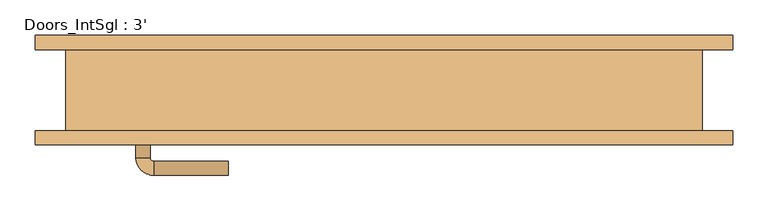
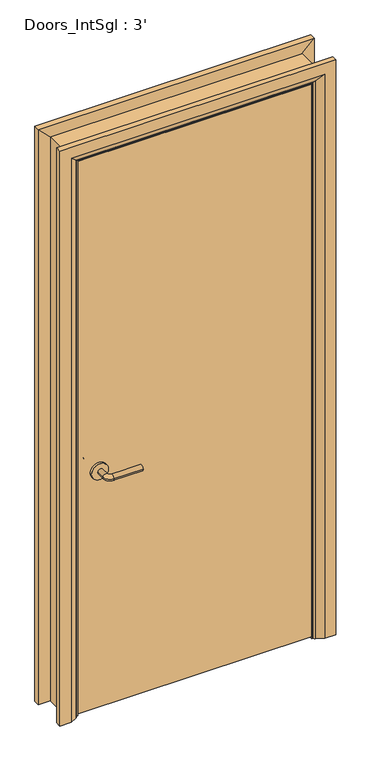
"""IFC4 building model written with IfcOpenShell, lengths in millimetres: door geometry, Doors_IntSgl : 3'."""

from ifc_helpers import new_model, si_unit, point, frame, frame_2d, origin, place, context, project, spatial, polyline, circle_curve, ellipse_curve, trimmed, segment, composite_curve, outline, extrude, faceted_brep, source, transform, mapped, element, save
from ifc_brep_helpers import plane_surface, cylinder_surface, revolved_surface, advanced_brep


def doors_intsgl_3_f3216364(model_context):
    return source(origin(), model_context, "Body", "SolidModel", [
        advanced_brep(
        [(-350.2, -11.15, 900.0), (-330.2, -11.15, 900.0), (-350.2, 18.85, 900.0), (-330.2, 18.85, 900.0), (-325.2, 23.85, 900.0), (-325.2, 43.85, 900.0), (-220.2, 43.85, 900.0), (-220.2, 23.85, 900.0)],
        [
            (0, 1, circle_curve(frame((-340.2, -11.15, 900.0), z_axis=(0.0, -1.0, 0.0), x_axis=(1.0, 0.0, 0.0)), 10.0)),
            (1, 0, circle_curve(frame((-340.2, -11.15, 900.0), z_axis=(0.0, -1.0, 0.0), x_axis=(1.0, 0.0, 0.0)), 10.0)),
            (0, 2),
            (2, 3, circle_curve(frame((-340.2, 18.85, 900.0), z_axis=(0.0, -1.0, 0.0), x_axis=(1.0, 0.0, 0.0)), 10.0)),
            (3, 1),
            (3, 2, circle_curve(frame((-340.2, 18.85, 900.0), z_axis=(0.0, -1.0, 0.0), x_axis=(1.0, 0.0, 0.0)), 10.0)),
            (4, 3, circle_curve(frame((-325.2, 18.85, 900.0), z_axis=(0.0, 0.0, 1.0), x_axis=(-1.0, 0.0, 0.0)), 5.0)),
            (2, 5, circle_curve(frame((-325.2, 18.85, 900.0), z_axis=(0.0, 0.0, -1.0), x_axis=(-1.0, 0.0, 0.0)), 25.0)),
            (5, 4, circle_curve(frame((-325.2, 33.85, 900.0), z_axis=(-1.0, 0.0, 0.0), x_axis=(0.0, -1.0, 0.0)), 10.0)),
            (4, 5, circle_curve(frame((-325.2, 33.85, 900.0), z_axis=(-1.0, 0.0, 0.0), x_axis=(0.0, -1.0, 0.0)), 10.0)),
            (6, 7, circle_curve(frame((-220.2, 33.85, 900.0), z_axis=(1.0, 0.0, 0.0), x_axis=(0.0, -1.0, 0.0)), 10.0)),
            (7, 6, circle_curve(frame((-220.2, 33.85, 900.0), z_axis=(1.0, 0.0, 0.0), x_axis=(0.0, -1.0, 0.0)), 10.0)),
            (5, 6),
            (7, 4),
        ],
        [
            plane_surface(frame((-340.2, -11.15, 900.0), z_axis=(0.0, -1.0, 0.0), x_axis=(0.0, 0.0, 1.0))),
            cylinder_surface(frame((-340.2, -11.15, 900.0), z_axis=(0.0, -1.0, 0.0), x_axis=(1.0, 0.0, 0.0)), 10.0),
            revolved_surface(trimmed(ellipse_curve(frame((-340.2, 18.85, 900.0), z_axis=(0.0, -1.0, 0.0), x_axis=(1.0, 0.0, 0.0)), 10.0, 10.0), [point((-350.2, 18.85, 900.0))], [point((-330.2, 18.85, 900.0))], True, "CARTESIAN"), (-325.2, 18.85, 900.0), (0.0, 0.0, -1.0)),
            revolved_surface(trimmed(ellipse_curve(frame((-340.2, 18.85, 900.0), z_axis=(0.0, -1.0, 0.0), x_axis=(1.0, 0.0, 0.0)), 10.0, 10.0), [point((-330.2, 18.85, 900.0))], [point((-350.2, 18.85, 900.0))], True, "CARTESIAN"), (-325.2, 18.85, 900.0), (0.0, 0.0, -1.0)),
            plane_surface(frame((-220.2, 33.85, 900.0), z_axis=(1.0, 0.0, 0.0), x_axis=(0.0, 0.0, 1.0))),
            cylinder_surface(frame((-325.2, 33.85, 900.0), z_axis=(-1.0, 0.0, 0.0), x_axis=(0.0, -1.0, 0.0)), 10.0),
        ],
        [
            (0, [[1, 2]]),
            (1, [[-1, 3, 4, 5]]),
            (1, [[-2, -5, 6, -3]]),
            (2, [[7, -4, 8, 9]]),
            (3, [[-8, -6, -7, 10]]),
            (4, [[11, 12]]),
            (5, [[-9, 13, -12, 14]]),
            (5, [[-10, -14, -11, -13]]),
        ],
    ),
        extrude(outline(composite_curve([segment(trimmed(circle_curve(frame_2d((900.0, -342.7)), 30.0), [point((900.0, -372.7))], [point((900.0, -312.7))], False, "CARTESIAN"), True, "CONTINUOUS"), segment(trimmed(circle_curve(frame_2d((900.0, -342.7)), 30.0), [point((900.0, -312.7))], [point((900.0, -372.7))], False, "CARTESIAN"), True, "CONTINUOUS")], self_intersect=False)), frame((0.0, -19.15, 0.0), z_axis=(0.0, 1.0, 0.0), x_axis=(0.0, 0.0, 1.0)), (0.0, 0.0, 1.0), 8.0),
        advanced_brep(
        [(-350.2, -65.15, 900.0), (-330.2, -65.15, 900.0), (-330.2, -95.15, 900.0), (-350.2, -95.15, 900.0), (-325.2, -100.15, 900.0), (-325.2, -120.15, 900.0), (-220.2, -120.15, 900.0), (-220.2, -100.15, 900.0)],
        [
            (0, 1, circle_curve(frame((-340.2, -65.15, 900.0), z_axis=(0.0, 1.0, 0.0), x_axis=(1.0, 0.0, 0.0)), 10.0)),
            (1, 0, circle_curve(frame((-340.2, -65.15, 900.0), z_axis=(0.0, 1.0, 0.0), x_axis=(1.0, 0.0, 0.0)), 10.0)),
            (1, 2),
            (2, 3, circle_curve(frame((-340.2, -95.15, 900.0), z_axis=(0.0, 1.0, 0.0), x_axis=(1.0, 0.0, 0.0)), 10.0)),
            (3, 0),
            (3, 2, circle_curve(frame((-340.2, -95.15, 900.0), z_axis=(0.0, 1.0, 0.0), x_axis=(1.0, 0.0, 0.0)), 10.0)),
            (4, 5, circle_curve(frame((-325.2, -110.15, 900.0), z_axis=(-1.0, 0.0, 0.0), x_axis=(0.0, 1.0, 0.0)), 10.0)),
            (5, 3, circle_curve(frame((-325.2, -95.15, 900.0), z_axis=(0.0, 0.0, -1.0), x_axis=(-1.0, 0.0, 0.0)), 25.0)),
            (2, 4, circle_curve(frame((-325.2, -95.15, 900.0), z_axis=(0.0, 0.0, 1.0), x_axis=(-1.0, 0.0, 0.0)), 5.0)),
            (5, 4, circle_curve(frame((-325.2, -110.15, 900.0), z_axis=(-1.0, 0.0, 0.0), x_axis=(0.0, 1.0, 0.0)), 10.0)),
            (6, 7, circle_curve(frame((-220.2, -110.15, 900.0), z_axis=(1.0, 0.0, 0.0), x_axis=(0.0, 1.0, 0.0)), 10.0)),
            (7, 6, circle_curve(frame((-220.2, -110.15, 900.0), z_axis=(1.0, 0.0, 0.0), x_axis=(0.0, 1.0, 0.0)), 10.0)),
            (4, 7),
            (6, 5),
        ],
        [
            plane_surface(frame((-340.2, -65.15, 900.0), z_axis=(0.0, 1.0, 0.0), x_axis=(0.0, 0.0, 1.0))),
            cylinder_surface(frame((-340.2, -65.15, 900.0), z_axis=(0.0, 1.0, 0.0), x_axis=(1.0, 0.0, 0.0)), 10.0),
            revolved_surface(trimmed(ellipse_curve(frame((-340.2, -95.15, 900.0), z_axis=(0.0, -1.0, 0.0), x_axis=(1.0, 0.0, 0.0)), 10.0, 10.0), [point((-350.2, -95.15, 900.0))], [point((-330.2, -95.15, 900.0))], True, "CARTESIAN"), (-325.2, -95.15, 900.0), (0.0, 0.0, -1.0)),
            revolved_surface(trimmed(ellipse_curve(frame((-340.2, -95.15, 900.0), z_axis=(0.0, -1.0, 0.0), x_axis=(1.0, 0.0, 0.0)), 10.0, 10.0), [point((-330.2, -95.15, 900.0))], [point((-350.2, -95.15, 900.0))], True, "CARTESIAN"), (-325.2, -95.15, 900.0), (0.0, 0.0, -1.0)),
            plane_surface(frame((-220.2, -110.15, 900.0), z_axis=(1.0, 0.0, 0.0), x_axis=(0.0, 0.0, 1.0))),
            cylinder_surface(frame((-325.2, -110.15, 900.0), z_axis=(-1.0, 0.0, 0.0), x_axis=(0.0, 1.0, 0.0)), 10.0),
        ],
        [
            (0, [[1, 2]]),
            (1, [[3, 4, 5, -2]]),
            (1, [[-5, 6, -3, -1]]),
            (2, [[7, 8, -4, 9]]),
            (3, [[10, -9, -6, -8]]),
            (4, [[11, 12]]),
            (5, [[13, -11, 14, -7]]),
            (5, [[-14, -12, -13, -10]]),
        ],
    ),
        extrude(outline(composite_curve([segment(trimmed(circle_curve(frame_2d((900.0, -342.7)), 30.0), [point((900.0, -372.7))], [point((900.0, -312.7))], False, "CARTESIAN"), True, "CONTINUOUS"), segment(trimmed(circle_curve(frame_2d((900.0, -342.7)), 30.0), [point((900.0, -312.7))], [point((900.0, -372.7))], False, "CARTESIAN"), True, "CONTINUOUS")], self_intersect=False)), frame((0.0, -65.15, 0.0), z_axis=(0.0, 1.0, 0.0), x_axis=(0.0, 0.0, 1.0)), (0.0, 0.0, 1.0), 8.0),
        extrude(outline(polyline([(415.2, -19.15), (415.2, -57.15), (-415.2, -57.15), (-415.2, -19.15), (415.2, -19.15)])), frame((0.0, 0.0, 8.0), z_axis=(0.0, 0.0, 1.0), x_axis=(1.0, 0.0, 0.0)), (0.0, 0.0, 1.0), 2083.6),
        advanced_brep(
        [(492.2, -77.15, 0.0), (452.2, -77.15, 0.0), (426.2, -63.15, 0.0), (422.2, -57.15, 0.0), (492.2, -57.15, 0.0), (492.2, -57.15, 2168.6), (492.2, -77.15, 2168.6), (422.2, -57.15, 2098.6), (-422.2, -57.15, 2098.6), (-422.2, -57.15, 0.0), (-492.2, -57.15, 0.0), (-492.2, -57.15, 2168.6), (426.2, -63.15, 2102.6), (452.2, -77.15, 2128.6), (-492.2, -77.15, 2168.6), (-492.2, -77.15, 0.0), (-452.2, -77.15, 0.0), (-452.2, -77.15, 2128.6), (-426.2, -63.15, 0.0), (-426.2, -63.15, 2102.6)],
        [
            (0, 1),
            (1, 2),
            (2, 3, circle_curve(frame((430.2, -56.15, 0.0), z_axis=(0.0, 0.0, -1.0), x_axis=(1.0, 0.0, 0.0)), 8.0622577)),
            (3, 4),
            (4, 0),
            (4, 5),
            (5, 6),
            (6, 0),
            (3, 7),
            (7, 8),
            (8, 9),
            (9, 10),
            (10, 11),
            (11, 5),
            (2, 12),
            (12, 7, ellipse_curve(frame((430.2, -56.15, 2106.6), z_axis=(0.7071067811865475, 0.0, -0.7071067811865475), x_axis=(-0.7071067811865474, 0.0, -0.7071067811865476)), 11.4017543, 8.0622577)),
            (1, 13),
            (13, 12),
            (6, 14),
            (14, 15),
            (15, 16),
            (16, 17),
            (17, 13),
            (10, 15),
            (14, 11),
            (9, 18, circle_curve(frame((-430.2, -56.15, 0.0), z_axis=(0.0, 0.0, -1.0), x_axis=(-1.0, 0.0, 0.0)), 8.0622577)),
            (18, 16),
            (19, 18),
            (8, 19, ellipse_curve(frame((-430.2, -56.15, 2106.6), z_axis=(-0.7071067811865475, 0.0, -0.7071067811865475), x_axis=(-0.7071067811865474, 0.0, 0.7071067811865476)), 11.4017543, 8.0622577)),
            (19, 17),
            (12, 19),
        ],
        [
            plane_surface(frame((422.2, -57.15, 0.0), z_axis=(0.0, 0.0, -1.0), x_axis=(0.0, 1.0, 0.0))),
            plane_surface(frame((492.2, -77.15, 0.0), z_axis=(1.0, 0.0, 0.0), x_axis=(0.0, 0.0, 1.0))),
            plane_surface(frame((492.2, -57.15, 0.0), z_axis=(0.0, 1.0, 0.0), x_axis=(0.0, 0.0, 1.0))),
            cylinder_surface(frame((430.2, -56.15, 0.0), z_axis=(0.0, 0.0, -1.0), x_axis=(1.0, 0.0, 0.0)), 8.0622577),
            plane_surface(frame((426.2, -63.15, 0.0), z_axis=(-0.4740998230350126, -0.880471099922178, 0.0), x_axis=(0.0, 0.0, 1.0))),
            plane_surface(frame((452.2, -77.15, 0.0), z_axis=(0.0, -1.0, 0.0), x_axis=(0.0, 0.0, 1.0))),
            plane_surface(frame((-492.2, -77.15, 2168.6), z_axis=(-1.0, 0.0, 0.0), x_axis=(0.0, 0.0, -1.0))),
            plane_surface(frame((-422.2, -57.15, 0.0), z_axis=(0.0, 0.0, -1.0), x_axis=(0.0, 1.0, 0.0))),
            cylinder_surface(frame((-430.2, -56.15, 2098.6), z_axis=(0.0, 0.0, 1.0), x_axis=(-1.0, 0.0, 0.0)), 8.0622577),
            plane_surface(frame((-426.2, -63.15, 2102.6), z_axis=(0.47409982303501824, -0.8804710999221749, 0.0), x_axis=(0.0, 0.0, -1.0))),
            plane_surface(frame((492.2, -77.15, 2168.6), z_axis=(0.0, 0.0, 1.0), x_axis=(-1.0, 0.0, 0.0))),
            cylinder_surface(frame((422.2, -56.15, 2106.6), z_axis=(1.0, 0.0, 0.0), x_axis=(0.0, 0.0, 1.0)), 8.0622577),
            plane_surface(frame((426.2, -63.15, 2102.6), z_axis=(0.0, -0.8804710999221764, -0.4740998230350154), x_axis=(-1.0, 0.0, 0.0))),
        ],
        [
            (0, [[1, 2, 3, 4, 5]]),
            (1, [[6, 7, 8, -5]]),
            (2, [[9, 10, 11, 12, 13, 14, -6, -4]]),
            (3, [[15, 16, -9, -3]]),
            (4, [[17, 18, -15, -2]]),
            (5, [[-8, 19, 20, 21, 22, 23, -17, -1]]),
            (6, [[-13, 24, -20, 25]]),
            (7, [[-24, -12, 26, 27, -21]]),
            (8, [[28, -26, -11, 29]]),
            (9, [[-22, -27, -28, 30]]),
            (10, [[-14, -25, -19, -7]]),
            (11, [[31, -29, -10, -16]]),
            (12, [[-23, -30, -31, -18]]),
        ],
    ),
        extrude(outline(polyline([(0.0, -398.2), (2074.6, -398.2), (2074.6, 398.2), (0.0, 398.2), (0.0, 417.2), (2093.6, 417.2), (2093.6, -417.2), (0.0, -417.2), (0.0, -398.2)])), frame((0.0, -17.15, 0.0), z_axis=(0.0, 1.0, 0.0), x_axis=(0.0, 0.0, 1.0)), (0.0, 0.0, 1.0), 32.0),
        advanced_brep(
        [(-492.2, 77.15, 0.0), (-452.2, 77.15, 0.0), (-426.2, 63.15, 0.0), (-422.2, 57.15, 0.0), (-492.2, 57.15, 0.0), (-492.2, 57.15, 2168.6), (-492.2, 77.15, 2168.6), (-422.2, 57.15, 2098.6), (-426.2, 63.15, 2102.6), (-452.2, 77.15, 2128.6), (492.2, 77.15, 0.0), (492.2, 57.15, 0.0), (422.2, 57.15, 0.0), (426.2, 63.15, 0.0), (452.2, 77.15, 0.0), (492.2, 77.15, 2168.6), (452.2, 77.15, 2128.6), (426.2, 63.15, 2102.6), (422.2, 57.15, 2098.6), (492.2, 57.15, 2168.6)],
        [
            (0, 1),
            (1, 2),
            (2, 3, circle_curve(frame((-430.2, 56.15, 0.0), z_axis=(0.0, 0.0, -1.0), x_axis=(-1.0, 0.0, 0.0)), 8.0622577)),
            (3, 4),
            (4, 0),
            (4, 5),
            (5, 6),
            (6, 0),
            (3, 7),
            (7, 5),
            (2, 8),
            (8, 7, ellipse_curve(frame((-430.2, 56.15, 2106.6), z_axis=(-0.7071067811865475, 0.0, -0.7071067811865475), x_axis=(0.7071067811865474, 0.0, -0.7071067811865476)), 11.4017543, 8.0622577)),
            (1, 9),
            (9, 8),
            (6, 9),
            (10, 11),
            (11, 12),
            (12, 13, circle_curve(frame((430.2, 56.15, 0.0), z_axis=(0.0, 0.0, -1.0), x_axis=(1.0, 0.0, 0.0)), 8.0622577)),
            (13, 14),
            (14, 10),
            (15, 10),
            (14, 16),
            (16, 15),
            (13, 17),
            (17, 16),
            (12, 18),
            (18, 17, ellipse_curve(frame((430.2, 56.15, 2106.6), z_axis=(0.7071067811865475, 0.0, -0.7071067811865475), x_axis=(0.7071067811865474, 0.0, 0.7071067811865476)), 11.4017543, 8.0622577)),
            (11, 19),
            (19, 18),
            (15, 19),
            (5, 19),
            (15, 6),
            (7, 18),
            (8, 17),
            (9, 16),
        ],
        [
            plane_surface(frame((-422.2, 129.9510989, 0.0), z_axis=(0.0, 0.0, -1.0), x_axis=(1.0, 0.0, 0.0))),
            plane_surface(frame((-492.2, 77.15, 0.0), z_axis=(-1.0, 0.0, 0.0), x_axis=(0.0, 0.0, 1.0))),
            plane_surface(frame((-492.2, 57.15, 0.0), z_axis=(0.0, -1.0, 0.0), x_axis=(0.0, 0.0, 1.0))),
            cylinder_surface(frame((-430.2, 56.15, 0.0), z_axis=(0.0, 0.0, -1.0), x_axis=(-1.0, 0.0, 0.0)), 8.0622577),
            plane_surface(frame((-426.2, 63.15, 0.0), z_axis=(0.4740998230350183, 0.8804710999221749, 0.0), x_axis=(0.0, 0.0, 1.0))),
            plane_surface(frame((-452.2, 77.15, 0.0), z_axis=(0.0, 1.0, 0.0), x_axis=(0.0, 0.0, 1.0))),
            plane_surface(frame((422.2, 129.9510989, 0.0), z_axis=(0.0, 0.0, -1.0), x_axis=(-1.0, 0.0, 0.0))),
            plane_surface(frame((452.2, 77.15, 2128.6), z_axis=(0.0, 1.0, 0.0), x_axis=(0.0, 0.0, -1.0))),
            plane_surface(frame((426.2, 63.15, 2102.6), z_axis=(-0.4740998230350183, 0.8804710999221749, 0.0), x_axis=(0.0, 0.0, -1.0))),
            cylinder_surface(frame((430.2, 56.15, 2098.6), z_axis=(0.0, 0.0, 1.0), x_axis=(1.0, 0.0, 0.0)), 8.0622577),
            plane_surface(frame((492.2, 57.15, 2168.6), z_axis=(0.0, -1.0, 0.0), x_axis=(0.0, 0.0, -1.0))),
            plane_surface(frame((492.2, 77.15, 2168.6), z_axis=(1.0, 0.0, 0.0), x_axis=(0.0, 0.0, -1.0))),
            plane_surface(frame((-492.2, 77.15, 2168.6), z_axis=(0.0, 0.0, 1.0), x_axis=(1.0, 0.0, 0.0))),
            plane_surface(frame((-492.2, 57.15, 2168.6), z_axis=(0.0, -1.0, 0.0), x_axis=(1.0, 0.0, 0.0))),
            cylinder_surface(frame((-422.2, 56.15, 2106.6), z_axis=(-1.0, 0.0, 0.0), x_axis=(0.0, 0.0, 1.0)), 8.0622577),
            plane_surface(frame((-426.2, 63.15, 2102.6), z_axis=(0.0, 0.8804710999221749, -0.4740998230350183), x_axis=(1.0, 0.0, 0.0))),
            plane_surface(frame((-452.2, 77.15, 2128.6), z_axis=(0.0, 1.0, 0.0), x_axis=(1.0, 0.0, 0.0))),
        ],
        [
            (0, [[1, 2, 3, 4, 5]]),
            (1, [[6, 7, 8, -5]]),
            (2, [[9, 10, -6, -4]]),
            (3, [[11, 12, -9, -3]]),
            (4, [[13, 14, -11, -2]]),
            (5, [[-8, 15, -13, -1]]),
            (6, [[16, 17, 18, 19, 20]]),
            (7, [[21, -20, 22, 23]]),
            (8, [[-22, -19, 24, 25]]),
            (9, [[-24, -18, 26, 27]]),
            (10, [[-26, -17, 28, 29]]),
            (11, [[-28, -16, -21, 30]]),
            (12, [[31, -30, 32, -7]]),
            (13, [[33, -29, -31, -10]]),
            (14, [[34, -27, -33, -12]]),
            (15, [[35, -25, -34, -14]]),
            (16, [[-32, -23, -35, -15]]),
        ],
    ),
        faceted_brep([(-417.2, -57.15, 0.0), (-449.2, -57.15, 0.0), (-449.2, 57.15, 0.0), (-417.2, 57.15, 0.0), (-417.2, 57.15, 2093.6), (-417.2, -57.15, 2093.6), (-449.2, 57.15, 2125.6), (-449.2, -57.15, 2125.6), (417.2, -57.15, 0.0), (417.2, 57.15, 0.0), (449.2, 57.15, 0.0), (449.2, -57.15, 0.0), (417.2, -57.15, 2093.6), (449.2, -57.15, 2125.6), (449.2, 57.15, 2125.6), (417.2, 57.15, 2093.6)], [[[0, 1, 2, 3]], [[3, 4, 5, 0]], [[2, 6, 4, 3]], [[1, 7, 6, 2]], [[0, 5, 7, 1]], [[8, 9, 10, 11]], [[12, 8, 11, 13]], [[13, 11, 10, 14]], [[14, 10, 9, 15]], [[15, 9, 8, 12]], [[4, 15, 12, 5]], [[6, 14, 15, 4]], [[7, 13, 14, 6]], [[5, 12, 13, 7]]]),
    ])


if __name__ == "__main__":
    model = new_model("IFC4")
    model_context = context("Model", 3, world=origin())
    ifc_project = project(units=[si_unit("LENGTHUNIT", "METRE", prefix="MILLI")], contexts=[model_context])
    site = spatial("IfcSite", under=ifc_project)
    building = spatial("IfcBuilding", under=site)
    placement = place(None, origin())
    doors_intsgl_3_shape = doors_intsgl_3_f3216364(model_context)
    element("IfcDoor", 1, ObjectType="Doors_IntSgl : 3'", at=placement, inside=building, context=model_context, shape_type="MappedRepresentation", body=[
        mapped(doors_intsgl_3_shape, transform((0.0, 0.0, 0.0), x_axis=(1.0, 0.0, 0.0), y_axis=(0.0, 1.0, 0.0), z_axis=(0.0, 0.0, 1.0))),
    ])
    save(model, "model.ifc")

# Revit data of these elements
# Type "Doors_IntSgl : 3'"
#   Type Mark = "47"
#   Type Comments = "Internal Single"
#   Operation = "SingleSwingRight"
#   Manufacturer = "Revit"
#   Keynote = "L20"
#   Description = "Internal Single Door"
#   Analytic Construction = "Metal"
#   UnderCut = 0' - 0.31496"
#   Tolerance = 0' - 0.07874"
#   Thickness = 0' - 1.49606"
#   Thermal Resistance (R) = 0.270117 (m²·K)/W
#   Structural Tolerance = 0' - 0.31496"
#   StopDepth = 0' - 1.25984"
#   Stop Thickness = 0' - 0.74803"
#   Rough Width = 3' - 0"
#   Rough Height = 7' - 0"
#   Height to Top Lock Rail = 3' - 3.37008"
#   Heat Transfer Coefficient (U) = 3.7021 W/(m²·K)
#   Handle Z Distance = 2' - 11.43307"
#   Handle X Distance = 0' - 2.95276"
#   Frame Thickness = 0' - 1.25984"
#   Door Panel Width = 2' - 8.69291"
#   Door Panel Thickness = 0' - 1.49606"
#   Door Panel Offset = 0' - 0"
#   Height = 7' - 0"
#   Width = 3' - 0"
#   Door Panel Height = 6' - 10.0315"
#   Architrave Setback = 0' - 0.19685"
#   Vis - Ironmongery = yes
#   Material Ironmongery = Door - Handle
#   Material Frame = Door - Frame/Mullion (1)
#   Material Door = Door - Panel
#   Material Architrave = Door - Architrave
#   Visual Light Transmittance = 0
#   Solar Heat Gain Coefficient = 0
#   Function = (empty or 0)
#   Wall Closure = (empty or 0)
# Element 1 (IfcDoor, "Doors_IntSgl : 3'")
#   Materials on its faces: "Door - Architrave", "Door - Handle", "Door - Frame/Mullion (1)", "Door - Panel"
# Materials
#   "Door - Handle": colour RGB 0 0 0, transparency 0, Keynote = "P21", Cost = 0
#   "Door - Frame/Mullion (1)": class "Wood", colour RGB 212 179 113, transparency 0, Keynote = "L20", Cost = 0
#   "Door - Panel": class "Wood", colour RGB 210 159 95, transparency 0, Keynote = "L20", Cost = 0
#   "Door - Architrave": class "Wood", colour RGB 154 90 5, transparency 0, Keynote = "P20", Cost = 0
